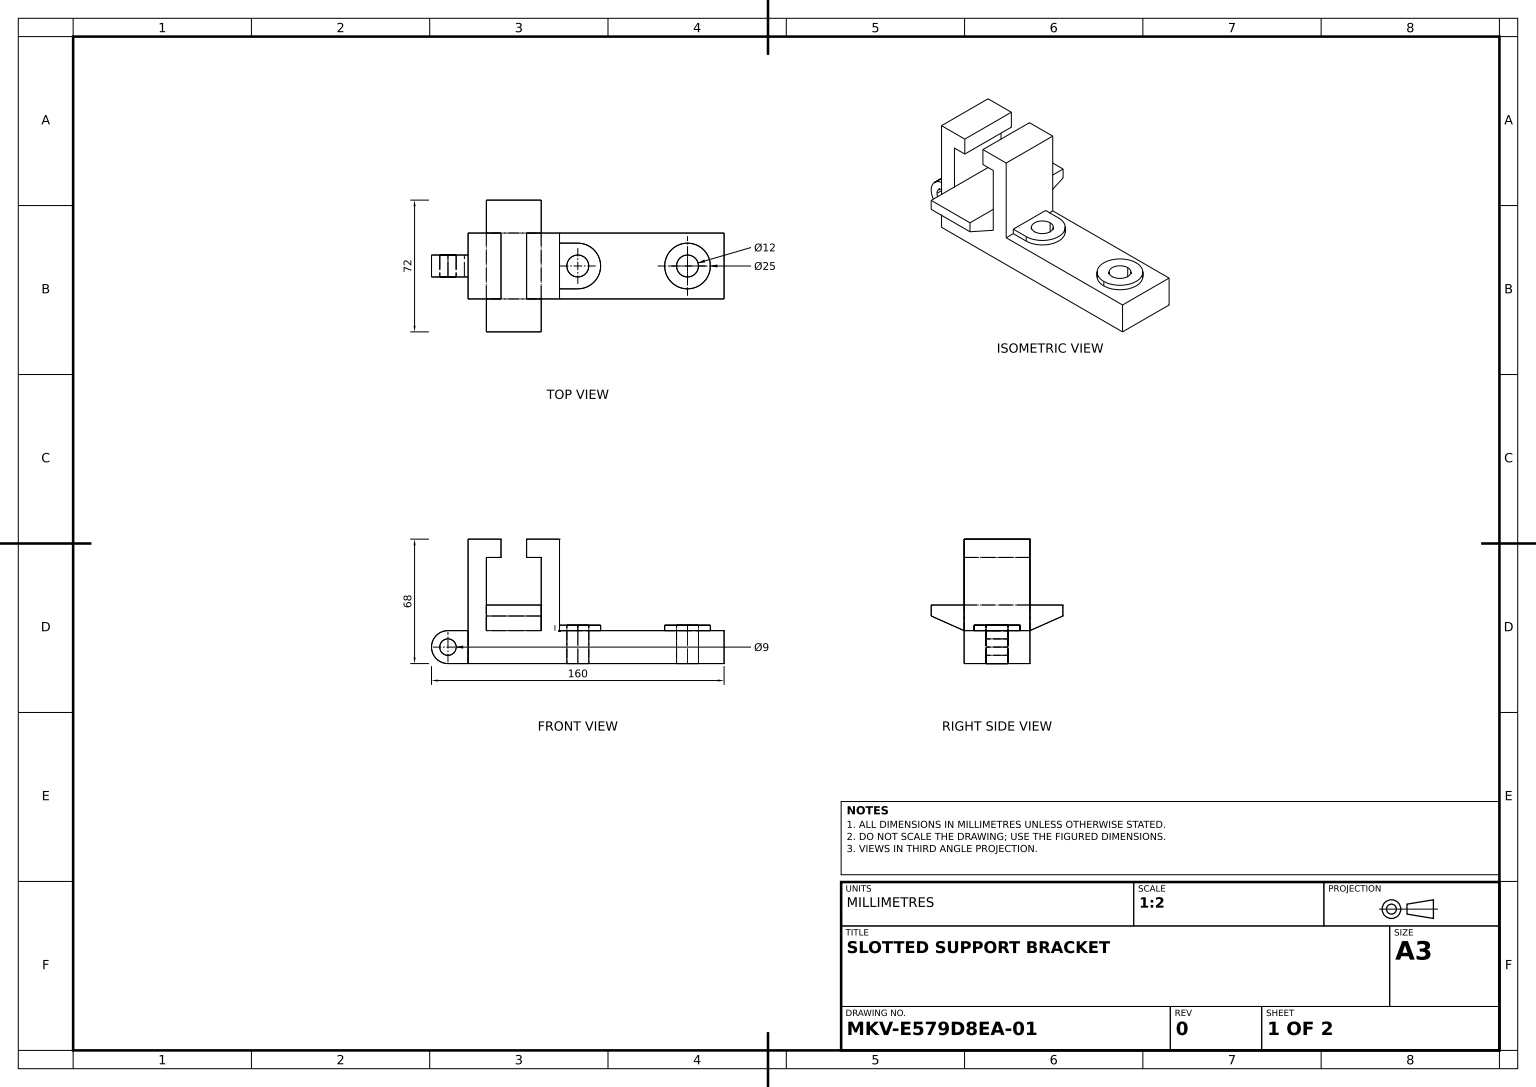
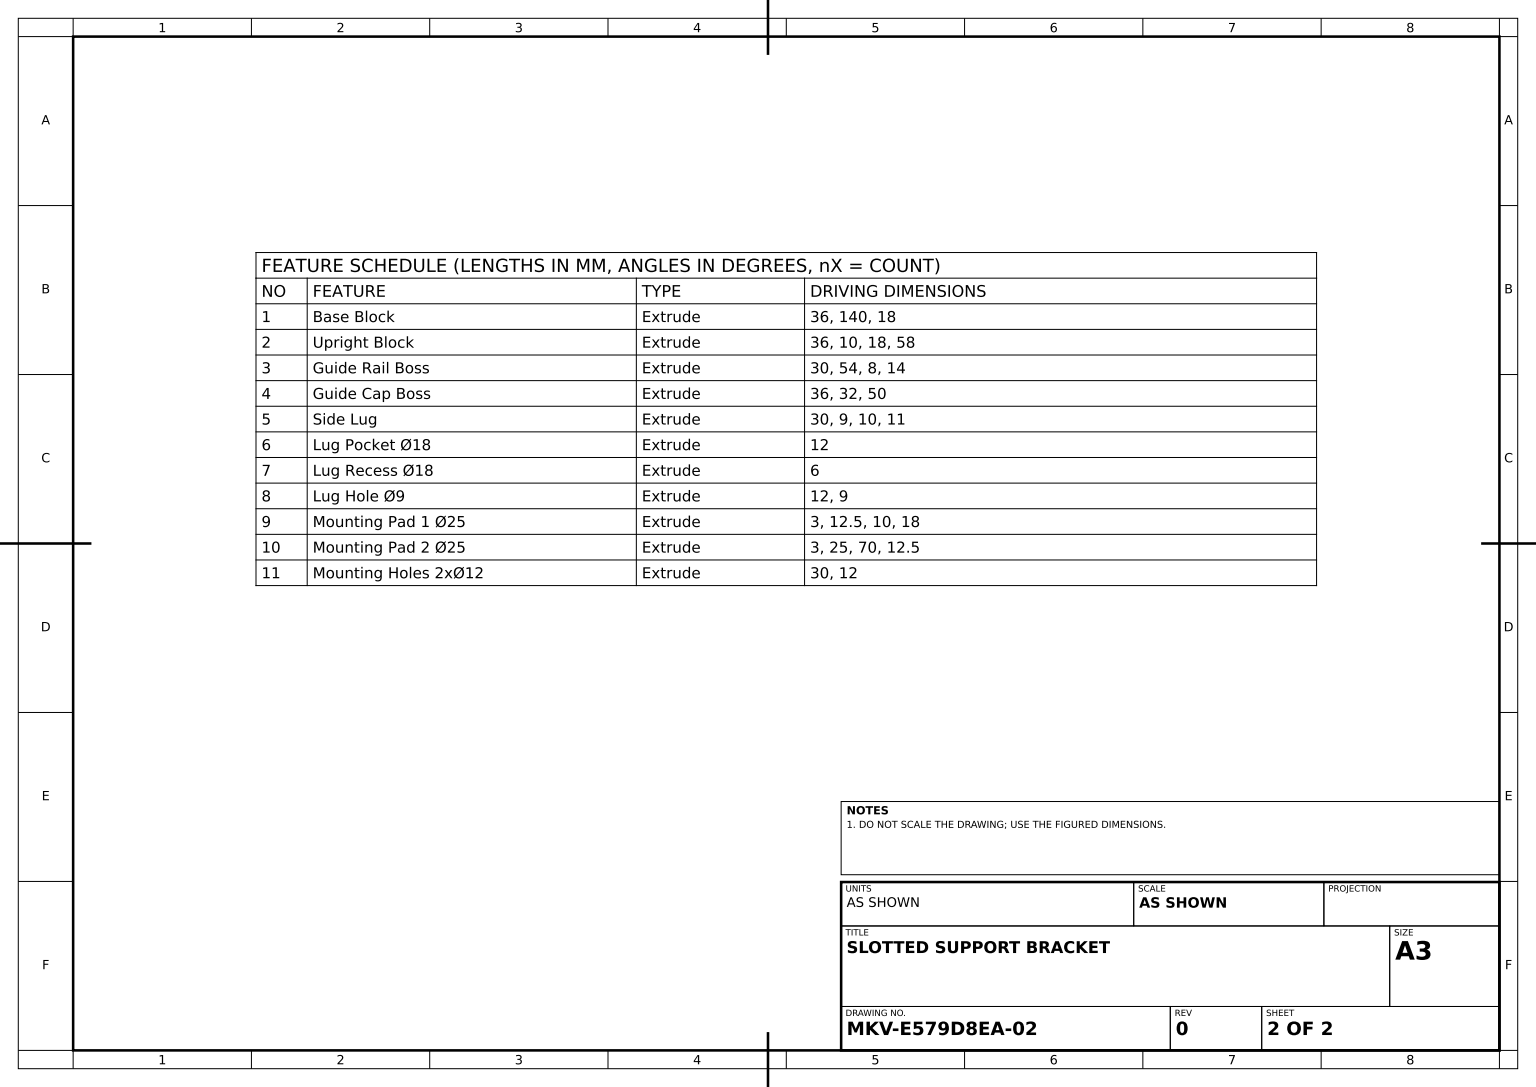
SolidWorks part; units mm, degrees
material "Plain Carbon Steel"
ref_plane "Front Plane" through (0, 0, 0) normal (0, 0, 1) x (1, 0, 0)
ref_plane "Top Plane" through (0, 0, 0) normal (0, 1, 0) x (1, 0, 0)
ref_plane "Right Plane" through (0, 0, 0) normal (1, 0, 0) x (0, 0, -1)
sketch "Base Profile Sketch" plane through (0, 0, 0) normal (0, 0, 1) x (1, 0, 0)
  line L0 (0, 0) -> (140, 0)
  line L1 (140, 0) -> (140, 18)
  line L2 (140, 18) -> (0, 18)
  line L3 (0, 18) -> (0, 0)
  dimension "D1" = 140
  dimension "D2" = 18
extrude "Base Block" add sketch "Base Profile Sketch" along normal blind 36
sketch "Upright Profile Sketch" plane through (0, 0, 36) normal (0, 0, 1) x (1, 0, 0)
  line L0 (0, 18) -> (0, 68)
  line L1 (0, 68) -> (18, 68)
  line L4 (18, 68) -> (18, 58)
  line L6 (0, 18) -> (10, 18)
  line L7 (140, 18) -> (0, 18) construction
  line L8 (10, 18) -> (10, 58)
  line L9 (10, 58) -> (18, 58)
  line L10 (0, 18) -> (0, 0) construction
  line L11 (0, 0) -> (140, 0) construction
  dimension "D1" = 10
  dimension "D2" = 18
  dimension "D3" = 58
extrude "Upright Block" add sketch "Upright Profile Sketch" against normal blind 36
sketch "Guide Rail Sketch" plane through (10, 0, 0) normal (1, 0, 0) x (0, 0, -1)
  line L1 (-36, 18) -> (0, 18) construction
  line L2 (-18, 32) -> (18, 32)
  line L3 (18, 32) -> (18, 26)
  line L4 (18, 26) -> (0, 18)
  line L5 (0, 18) -> (-18, 18)
  line L6 (-18, 32) -> (-54, 32)
  line L7 (-54, 32) -> (-54, 26)
  line L8 (-54, 26) -> (-36, 18)
  line L9 (-36, 18) -> (-18, 18)
  line L10 (-36, 18) -> (-36, 58) construction
  line L11 (0, 18) -> (-36, 18) construction
  dimension "D1" = 54
  dimension "D2" = 8
  dimension "D3" = 14
extrude "Guide Rail Boss" add sketch "Guide Rail Sketch" along normal blind 30
sketch "Guide Cap Sketch" plane through (0, 0, 0) normal (0, 0, -1) x (-1, 0, 0)
  line L0 (-40, 18) -> (-50, 18)
  line L1 (-140, 18) -> (-40, 18) construction
  line L2 (-50, 18) -> (-50, 68)
  line L3 (-50, 68) -> (-32, 68)
  line L4 (-32, 68) -> (-32, 58)
  line L5 (-40, 18) -> (-40, 58)
  line L6 (-40, 58) -> (-32, 58)
  line L7 (0, 68) -> (0, 0) construction
  dimension "D1" = 32
  dimension "D2" = 50
extrude "Guide Cap Boss" add sketch "Guide Cap Sketch" against normal blind 36
sketch "Side Lug Sketch" plane through (0, 0, 0) normal (0, 0, -1) x (-1, 0, 0)
  line L0 (0, 0) -> (0, 18)
  line L1 (0, 68) -> (0, 0) construction
  line L2 (0, 18) -> (10, 18)
  line L3 (10, 18) -> (11, 18)
  line L5 (11, 0) -> (0, 0)
  arc A0 (11, 0) -> (11, 18) centre (11, 9) ccw
  dimension "D1" = 18
  dimension "D2" = 9
  dimension "D3" = 10
  dimension "D4" = 11
extrude "Side Lug" add sketch "Side Lug Sketch" against normal blind 30
sketch "Lug Pocket Sketch" plane through (0, 0, 0) normal (0, 0, -1) x (-1, 0, 0)
  line L0 (0, 18) -> (11, 18)
  line L2 (11, 0) -> (0, 0)
  line L3 (0, 0) -> (0, 18)
  arc A0 (11, 0) -> (11, 18) centre (11, 9) ccw
  dimension "D1" = 18
extrude "Lug Pocket Ø18" cut sketch "Lug Pocket Sketch" against normal blind 12
sketch "Lug Recess Sketch" plane through (0, 0, 30) normal (0, 0, 1) x (1, 0, 0)
  line L0 (0, 18) -> (-11, 18)
  line L2 (-11, 0) -> (0, 0)
  line L3 (0, 0) -> (0, 18)
  arc A0 (-11, 18) -> (-11, 0) centre (-11, 9) ccw construction
  arc A1 (-11, 18) -> (-11, 0) centre (-11, 9) ccw
  dimension "D1" = 18
extrude "Lug Recess Ø18" cut sketch "Lug Recess Sketch" against normal blind 6
sketch "Lug Hole Sketch" plane through (0, 0, 24) normal (0, 0, 1) x (1, 0, 0)
  circle A0 centre (-11, 9) radius 4.5
  dimension "D1" = 9
  dimension "D2" = 9
extrude "Lug Hole Ø9" cut sketch "Lug Hole Sketch" against normal blind 12
sketch "Mounting Pad 1 Sketch" plane through (0, 18, 0) normal (0, 1, 0) x (1, 0, 0)
  line L0 (140, 0) -> (50, 0) construction
  line L1 (50, -36) -> (50, 0) construction
  line L2 (60, -5.5) -> (50, -5.5)
  line L3 (50, -5.5) -> (50, -30.5)
  line L4 (50, -36) -> (50, 0) construction
  line L5 (50, -30.5) -> (60, -30.5)
  arc A0 (60, -30.5) -> (60, -5.5) centre (60, -18) ccw
  dimension "D1" = 25
  dimension "D2" = 12.5
  dimension "D3" = 10
  dimension "D4" = 18
extrude "Mounting Pad 1 Ø25" add sketch "Mounting Pad 1 Sketch" along normal blind 3
sketch "Mounting Pad 2 Sketch" plane through (0, 18, 0) normal (0, 1, 0) x (1, 0, 0)
  line L0 (50, -36) -> (50, -30.5) construction
  line L1 (50, -30.5) -> (60, -30.5) construction
  circle A0 centre (120, -18) radius 12.5
  dimension "D1" = 25
  dimension "D2" = 25
  dimension "D3" = 70
  dimension "D4" = 12.5
extrude "Mounting Pad 2 Ø25" add sketch "Mounting Pad 2 Sketch" along normal blind 3
sketch "Mounting Holes Sketch" plane through (0, 21, 0) normal (0, 1, 0) x (1, 0, 0)
  circle A0 centre (120, -18) radius 6
  circle A1 centre (60, -18) radius 6
  dimension "D1" = 12
  dimension "D2" = 12
  dimension "D3" = 12
extrude "Mounting Holes 2xØ12" cut sketch "Mounting Holes Sketch" against normal blind 30
